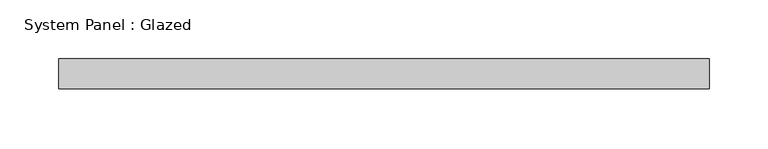
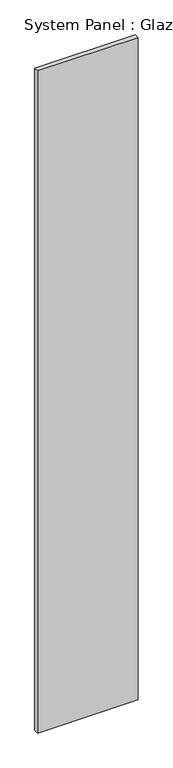
"""IFC4 building model written with IfcOpenShell, lengths in millimetres: plate geometry, System Panel : Glazed."""

from ifc_helpers import new_model, si_unit, origin, origin_with_axes, place, context, project, spatial, polyline, outline, extrude, source, transform, mapped, element, save


def system_panel_glazed_89573664(model_context):
    return source(origin(), model_context, "Body", "SweptSolid", [
        extrude(outline(polyline([(275.9422868, 19.05), (-275.9422868, 19.05), (-275.9422868, 44.45), (275.9422868, 44.45), (275.9422868, 19.05)])), origin_with_axes(), (0.0, 0.0, 1.0), 3835.4),
    ])


if __name__ == "__main__":
    model = new_model("IFC4")
    model_context = context("Model", 3, world=origin())
    ifc_project = project(units=[si_unit("LENGTHUNIT", "METRE", prefix="MILLI")], contexts=[model_context])
    site = spatial("IfcSite", under=ifc_project)
    building = spatial("IfcBuilding", under=site)
    placement = place(None, origin())
    system_panel_glazed_shape = system_panel_glazed_89573664(model_context)
    element("IfcPlate", 1, ObjectType="System Panel : Glazed", at=placement, inside=building, context=model_context, shape_type="MappedRepresentation", body=[
        mapped(system_panel_glazed_shape, transform((0.0, 0.0, 0.0), x_axis=(1.0, 0.0, 0.0), y_axis=(0.0, 1.0, 0.0), z_axis=(0.0, 0.0, 1.0))),
    ])
    save(model, "model.ifc")

# Revit data of these elements
# Type "System Panel : Glazed"
#   Construction Type Id = "GSP4R"
#   Analytic Construction = "1/8 in Pilkington single glazing"
#   Visual Light Transmittance = 0.9
#   Solar Heat Gain Coefficient = 0.86
#   Heat Transfer Coefficient (U) = 1.18115 BTU/(h·ft²·°F)
# Element 1 (IfcPlate, "System Panel : Glazed")
#   Materials on its faces: "Glass"
# Materials
#   "Glass": class "Glass", colour RGB 0 128 192, transparency 0.75, Description = "Soda Lime Glass", Cost = 0
